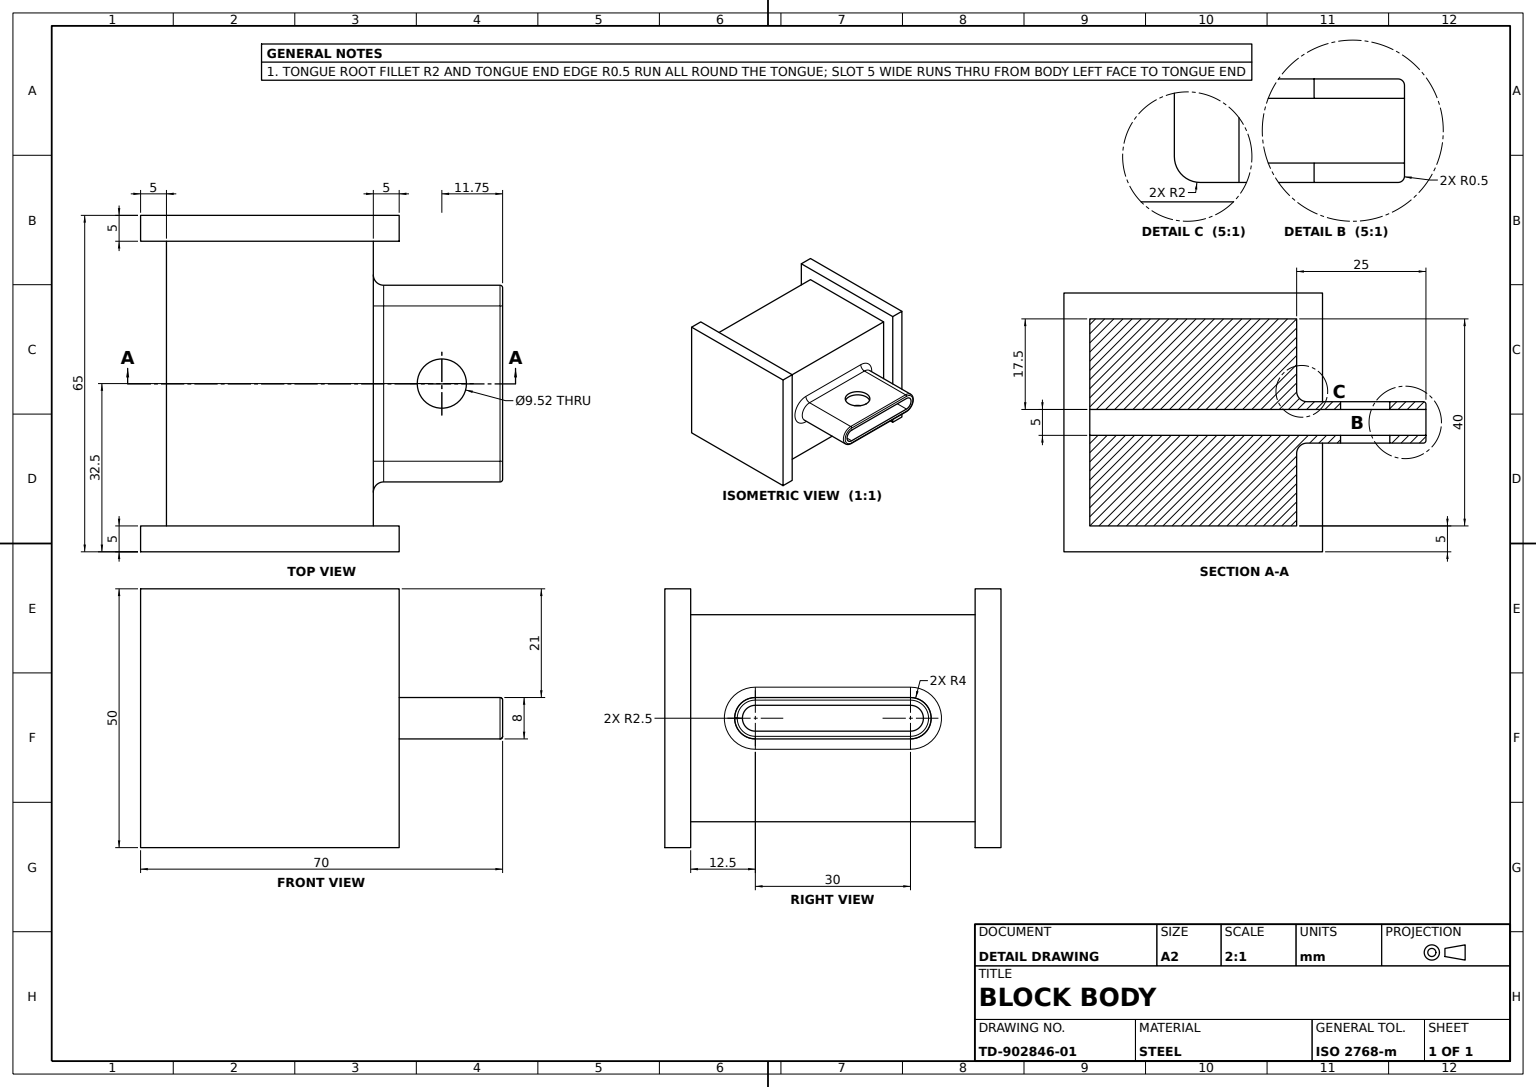
from build123d import *

# Parameters (mm, degrees)
FRONT_FLANGE_SKETCH_W      = 50
FRONT_FLANGE_SKETCH_H      = 50
FRONT_FLANGE_50X50X5_DEPTH = 5
BODY_BLOCK_SKETCH_W        = 40
BODY_BLOCK_SKETCH_H        = 40
BODY_BLOCK_40X40X55_DEPTH  = 55
REAR_FLANGE_SKETCH_W       = 50
REAR_FLANGE_SKETCH_H       = 50
REAR_FLANGE_5MM_DEPTH      = 5
OBROUND_TONGUE_DEPTH       = 25
TONGUE_SLOT_CUT_DEPTH      = 108.819293264
TONGUE_ROOT_FILLET_R2_R    = 2
TONGUE_EDGE_FILLET_R0_5_R  = 0.5
TONGUE_HOLE_SKETCH_R       = 4.75949031
TONGUE_CROSS_HOLE_DEPTH    = 100.829855254


with BuildPart() as part:
    # Front Flange Sketch → Front Flange 50x50x5 (new body)
    with BuildSketch(Plane.XY):
        with Locations((25, 25)):
            Rectangle(FRONT_FLANGE_SKETCH_W, FRONT_FLANGE_SKETCH_H)
    extrude(amount=FRONT_FLANGE_50X50X5_DEPTH)

    # Body Block Sketch → Body Block 40x40x55 (add)
    with BuildSketch(Plane.XY.offset(5)):
        with Locations((25, 25)):
            Rectangle(BODY_BLOCK_SKETCH_W, BODY_BLOCK_SKETCH_H)
    extrude(amount=BODY_BLOCK_40X40X55_DEPTH)

    # Rear Flange Sketch → Rear Flange 5mm (add)
    with BuildSketch(Plane.XY.offset(60)):
        with Locations((25, 25)):
            Rectangle(REAR_FLANGE_SKETCH_W, REAR_FLANGE_SKETCH_H)
    extrude(amount=REAR_FLANGE_5MM_DEPTH)

    # Tongue Profile Sketch → Obround Tongue (add)
    with BuildSketch(Plane(origin=(45, 0, 0), x_dir=(0, 0, -1), z_dir=(1, 0, 0))):
        with BuildLine():
            Line((-47.5, 29), (-17.5, 29))
            ThreePointArc((-17.5, 29), (-13.5, 25), (-17.5, 21))
            Line((-17.5, 21), (-47.5, 21))
            ThreePointArc((-47.5, 21), (-51.5, 25), (-47.5, 29))
        make_face()
    extrude(amount=OBROUND_TONGUE_DEPTH)

    # Tongue Slot Sketch → Tongue Slot Cut (cut, through all)
    with BuildSketch(Plane(origin=(70, 0, 0), x_dir=(0, 0, -1), z_dir=(1, 0, 0))):
        with BuildLine():
            Line((-47.5, 22.5), (-17.5, 22.5))
            ThreePointArc((-17.5, 22.5), (-15, 25), (-17.5, 27.5))
            Line((-17.5, 27.5), (-47.5, 27.5))
            ThreePointArc((-47.5, 27.5), (-50, 25), (-47.5, 22.5))
        make_face()
    extrude(amount=-TONGUE_SLOT_CUT_DEPTH, mode=Mode.SUBTRACT)

    # Tongue Root Fillet R2
    tongue_root_fillet_r2_edges = [part.edges().sort_by_distance(p)[0] for p in [
        (45, 29, 32.5),
        (45, 25, 13.5),
        (45, 21, 32.5),
        (45, 25, 51.5),
    ]]
    fillet(tongue_root_fillet_r2_edges, radius=TONGUE_ROOT_FILLET_R2_R)

    # Tongue Edge Fillet R0.5
    tongue_edge_fillet_r0_5_edges = [part.edges().sort_by_distance(p)[0] for p in [
        (70, 21, 32.5),
        (70, 25, 13.5),
        (70, 25, 51.5),
        (70, 29, 32.5),
    ]]
    fillet(tongue_edge_fillet_r0_5_edges, radius=TONGUE_EDGE_FILLET_R0_5_R)

    # Tongue Hole Sketch → Tongue Cross Hole (cut, through all)
    with BuildSketch(Plane.XZ.offset(-21)):
        with Locations((58.25, 32.5)):
            Circle(TONGUE_HOLE_SKETCH_R)
    extrude(amount=-TONGUE_CROSS_HOLE_DEPTH, mode=Mode.SUBTRACT)


solid = part.part
